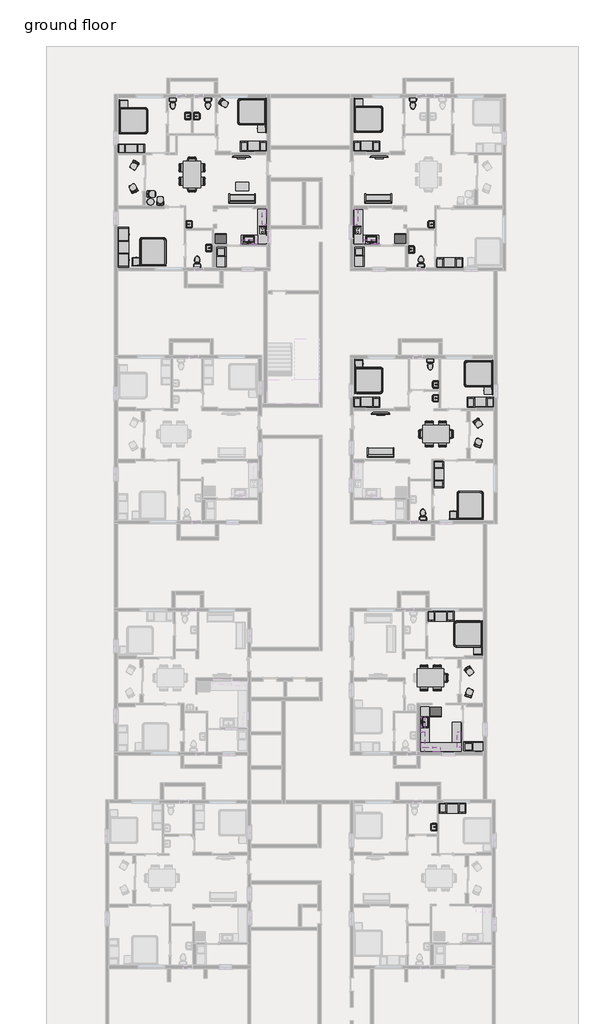
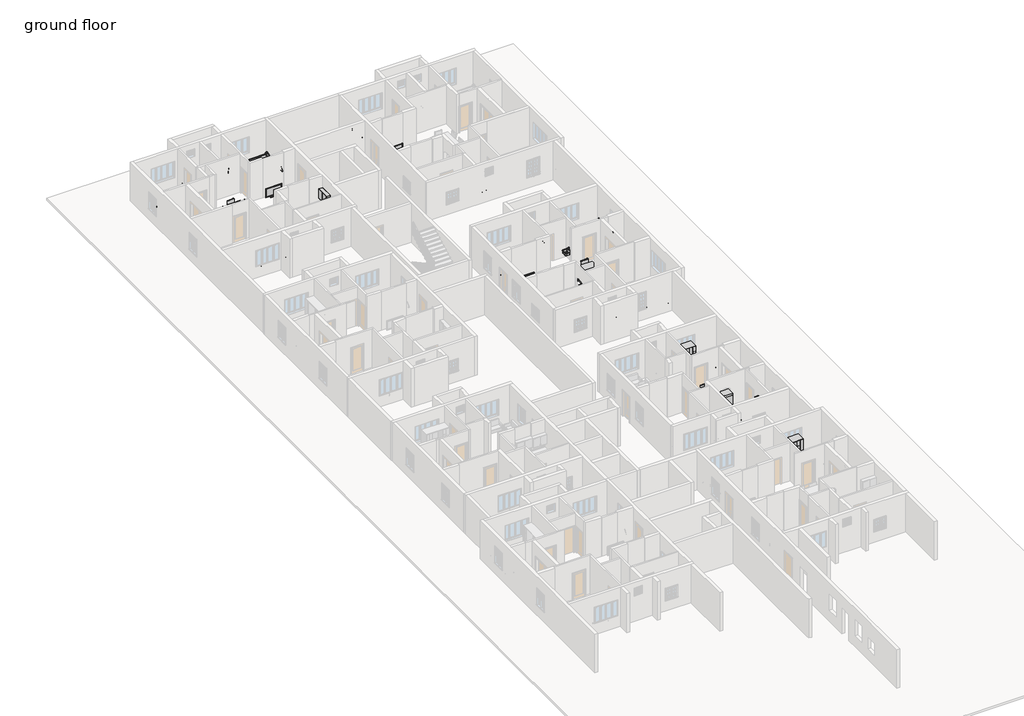
# One storey, part 13 of 16: 81 furniture elements, 19 flow terminals, 11 proxies.
"""IFC4 building model written with IfcOpenShell, lengths in millimetres."""

from ifc_helpers import new_model, si_unit, origin, place, context, project, spatial, transform, mapped, element, save
from components import proxy_84368fe0, proxy_40295e01, proxy_97c73763, proxy_19935bb1, proxy_76352e5b, proxy_1934c8a4, flow_terminal_4d548711, flow_terminal_3ac2e542, flow_terminal_8d9ea526, toilet_domestic_3d_toilet_domestic_3d_ba6479b0, toilet_domestic_3d_toilet_domestic_3d_30431060, bed_design_8999_bed_design_8999_9c973422, bed_design_8999_bed_design_8999_e911dec7, furniture_f87f75a4, furniture_a56de0b1, furniture_5ca60c7f, furniture_97fe820d, furniture_007fecef, chair_task_chair_task_b7f3823b, chair_task_arms_chair_task_arms_fa5a08ef, furniture_deb1c5d1, furniture_78fcf777, furniture_7591947b, furniture_03a15ce7, furniture_53e129a0, furniture_dd44345b, furniture_3d2ef6d7, furniture_88072bd9, furniture_1f19b6cd, furniture_eb3a3c23, furniture_4fdbbe14, furniture_57f9710a, furniture_0b81fedb, furniture_e479396c, furniture_0bcc43ae, furniture_9d41381f, furniture_9929ec1f, furniture_f73e1c42

model = new_model("IFC4")

# Units and contexts
model_context = context("Model", 3, world=origin())
ifc_project = project(units=[si_unit("LENGTHUNIT", "METRE", prefix="MILLI")], contexts=[model_context])

# Site, building, storey
site = spatial("IfcSite", under=ifc_project)
building = spatial("IfcBuilding", under=site)
storey = spatial("IfcBuildingStorey", under=building, Name="ground floor", Elevation=609.6)

# Proxies
placement = place(None, origin())
proxy_shape = proxy_84368fe0(model_context)
element("IfcBuildingElementProxy", 1, Name="Cook Top-2 Unit : 16\" x 22\"", ObjectType="Cook Top-2 Unit : 16\" x 22\"", at=placement, inside=storey, context=model_context, shape_type="MappedRepresentation", body=[
    mapped(proxy_shape, transform((53260.5312819, 41205.614288, 609.6), x_axis=(1.0, 0.0, 0.0), y_axis=(0.0, 1.0, 0.0), z_axis=(0.0, 0.0, 1.0))),
])
proxy_2_shape = proxy_40295e01(model_context)
element("IfcBuildingElementProxy", 2, Name="Cook Top-2 Unit : 16\" x 22\"", ObjectType="Cook Top-2 Unit : 16\" x 22\"", at=placement, inside=storey, context=model_context, shape_type="MappedRepresentation", body=[
    mapped(proxy_2_shape, transform((59966.1312819, 41205.614288, 609.6), x_axis=(-1.0, 0.0, 0.0), y_axis=(0.0, -1.0, 0.0), z_axis=(0.0, 0.0, 1.0))),
])
proxy_3_shape = proxy_97c73763(model_context)
element("IfcBuildingElementProxy", 3, Name="Dryer : 27\" x 25\" x 35\"", ObjectType="Dryer : 27\" x 25\" x 35\"", at=placement, inside=storey, context=model_context, shape_type="MappedRepresentation", body=[
    mapped(proxy_3_shape, transform((50190.0538966, 39449.1934981, 609.6), x_axis=(0.0, -1.0, 0.0), y_axis=(1.0, 0.0, 0.0), z_axis=(0.0, 0.0, 1.0))),
])
element("IfcBuildingElementProxy", 4, Name="Dryer : 27\" x 25\" x 35\"", ObjectType="Dryer : 27\" x 25\" x 35\"", at=placement, inside=storey, context=model_context, shape_type="MappedRepresentation", body=[
    mapped(proxy_3_shape, transform((59691.3278279, 39474.5934981, 609.6), x_axis=(0.0, -1.0, 0.0), y_axis=(1.0, 0.0, 0.0), z_axis=(0.0, 0.0, 1.0))),
])
element("IfcBuildingElementProxy", 5, Name="Dryer : 27\" x 25\" x 35\"", ObjectType="Dryer : 27\" x 25\" x 35\"", at=placement, inside=storey, context=model_context, shape_type="MappedRepresentation", body=[
    mapped(proxy_3_shape, transform((67812.0859463, 5399.7775766, 609.6), x_axis=(1.0, 0.0, 0.0), y_axis=(0.0, 1.0, 0.0), z_axis=(0.0, 0.0, 1.0))),
])
proxy_4_shape = proxy_19935bb1(model_context)
element("IfcBuildingElementProxy", 6, Name="Refrigerator-Built-in : 30\" x 24\" LH", ObjectType="Refrigerator-Built-in : 30\" x 24\" LH", at=placement, inside=storey, context=model_context, shape_type="MappedRepresentation", body=[
    mapped(proxy_4_shape, transform((65262.8133315, 8104.2496364, 609.6), x_axis=(1.0, 0.0, 0.0), y_axis=(0.0, 1.0, 0.0), z_axis=(0.0, 0.0, 1.0))),
])
proxy_5_shape = proxy_76352e5b(model_context)
element("IfcBuildingElementProxy", 7, Name="Refrigerator-Built-in : 30\" x 24\" LH", ObjectType="Refrigerator-Built-in : 30\" x 24\" LH", at=placement, inside=storey, context=model_context, shape_type="MappedRepresentation", body=[
    mapped(proxy_5_shape, transform((50460.1812819, 40629.665558, 609.6), x_axis=(1.0, 0.0, 0.0), y_axis=(0.0, 1.0, 0.0), z_axis=(0.0, 0.0, 1.0))),
])
element("IfcBuildingElementProxy", 8, Name="Refrigerator-Built-in : 30\" x 24\" LH", ObjectType="Refrigerator-Built-in : 30\" x 24\" LH", at=placement, inside=storey, context=model_context, shape_type="MappedRepresentation", body=[
    mapped(proxy_5_shape, transform((62806.2552131, 40629.665558, 609.6), x_axis=(1.0, 0.0, 0.0), y_axis=(0.0, 1.0, 0.0), z_axis=(0.0, 0.0, 1.0))),
])
proxy_6_shape = proxy_1934c8a4(model_context)
element("IfcBuildingElementProxy", 9, Name="Washer : 25\" x 25\" x 35\"", ObjectType="Washer : 25\" x 25\" x 35\"", at=placement, inside=storey, context=model_context, shape_type="MappedRepresentation", body=[
    mapped(proxy_6_shape, transform((50225.5653356, 40125.6235103, 609.6), x_axis=(0.0, -1.0, 0.0), y_axis=(1.0, 0.0, 0.0), z_axis=(0.0, 0.0, 1.0))),
])
element("IfcBuildingElementProxy", 10, Name="Washer : 25\" x 25\" x 35\"", ObjectType="Washer : 25\" x 25\" x 35\"", at=placement, inside=storey, context=model_context, shape_type="MappedRepresentation", body=[
    mapped(proxy_6_shape, transform((59726.8392669, 40151.0235103, 609.6), x_axis=(0.0, -1.0, 0.0), y_axis=(1.0, 0.0, 0.0), z_axis=(0.0, 0.0, 1.0))),
])
element("IfcBuildingElementProxy", 11, Name="Washer : 25\" x 25\" x 35\"", ObjectType="Washer : 25\" x 25\" x 35\"", at=placement, inside=storey, context=model_context, shape_type="MappedRepresentation", body=[
    mapped(proxy_6_shape, transform((67110.9973853, 5441.2075888, 609.6), x_axis=(1.0, 0.0, 0.0), y_axis=(0.0, 1.0, 0.0), z_axis=(0.0, 0.0, 1.0))),
])

# Flow terminals
flow_terminal_shape = flow_terminal_4d548711(model_context)
element("IfcFlowTerminal", 12, ObjectType="Sink Kitchen-Single : 30\" x 21\"", at=placement, inside=storey, context=model_context, shape_type="MappedRepresentation", body=[
    mapped(flow_terminal_shape, transform((52412.6205224, 40563.7497039, 609.6), x_axis=(-1.0, 0.0, 0.0), y_axis=(0.0, -1.0, 0.0), z_axis=(0.0, 0.0, 1.0))),
])
element("IfcFlowTerminal", 13, ObjectType="Sink Kitchen-Single : 30\" x 21\"", at=placement, inside=storey, context=model_context, shape_type="MappedRepresentation", body=[
    mapped(flow_terminal_shape, transform((64489.676683, 7368.8508246, 609.6), x_axis=(0.0, 1.0, 0.0), y_axis=(-1.0, 0.0, 0.0), z_axis=(0.0, 0.0, 1.0))),
])
flow_terminal_2_shape = flow_terminal_3ac2e542(model_context)
element("IfcFlowTerminal", 14, ObjectType="Sink Kitchen-Single : 30\" x 21\"", at=placement, inside=storey, context=model_context, shape_type="MappedRepresentation", body=[
    mapped(flow_terminal_2_shape, transform((60814.0420413, 40563.7497039, 609.6), x_axis=(1.0, 0.0, 0.0), y_axis=(0.0, 1.0, 0.0), z_axis=(0.0, 0.0, 1.0))),
])
flow_terminal_3_shape = flow_terminal_8d9ea526(model_context)
element("IfcFlowTerminal", 15, ObjectType="Sink Vanity-Square : 20\" x 18\"", at=placement, inside=storey, context=model_context, shape_type="MappedRepresentation", body=[
    mapped(flow_terminal_3_shape, transform((48234.5058086, 41623.6015966, 609.6), x_axis=(0.01205714691658211, 0.9999273099621953, 0.0), y_axis=(-0.9999273099621953, 0.01205714691658211, 0.0), z_axis=(0.0, 0.0, 1.0))),
])
element("IfcFlowTerminal", 16, ObjectType="Sink Vanity-Square : 20\" x 18\"", at=placement, inside=storey, context=model_context, shape_type="MappedRepresentation", body=[
    mapped(flow_terminal_3_shape, transform((49691.1133168, 40018.2935434, 609.6), x_axis=(0.0, -1.0, 0.0), y_axis=(1.0, 0.0, 0.0), z_axis=(0.0, 0.0, 1.0))),
])
element("IfcFlowTerminal", 17, ObjectType="Sink Vanity-Square : 20\" x 18\"", at=placement, inside=storey, context=model_context, shape_type="MappedRepresentation", body=[
    mapped(flow_terminal_3_shape, transform((48245.9195817, 49103.029965, 609.6), x_axis=(0.0, -1.0, 0.0), y_axis=(1.0, 0.0, 0.0), z_axis=(0.0, 0.0, 1.0))),
])
element("IfcFlowTerminal", 18, ObjectType="Sink Vanity-Square : 20\" x 18\"", at=placement, inside=storey, context=model_context, shape_type="MappedRepresentation", body=[
    mapped(flow_terminal_3_shape, transform((48755.0527323, 49063.0030585, 609.6), x_axis=(0.0, 1.0, 0.0), y_axis=(-1.0, 0.0, 0.0), z_axis=(0.0, 0.0, 1.0))),
])
element("IfcFlowTerminal", 19, ObjectType="Sink Vanity-Square : 20\" x 18\"", at=placement, inside=storey, context=model_context, shape_type="MappedRepresentation", body=[
    mapped(flow_terminal_3_shape, transform((64991.9370405, 41653.02877, 609.6), x_axis=(0.0, -1.0, 0.0), y_axis=(1.0, 0.0, 0.0), z_axis=(0.0, 0.0, 1.0))),
])
element("IfcFlowTerminal", 20, ObjectType="Sink Vanity-Square : 20\" x 18\"", at=placement, inside=storey, context=model_context, shape_type="MappedRepresentation", body=[
    mapped(flow_terminal_3_shape, transform((63532.9943061, 39880.7582649, 609.6), x_axis=(-0.012057146916551579, 0.9999273099621956, 0.0), y_axis=(-0.9999273099621956, -0.012057146916551579, 0.0), z_axis=(0.0, 0.0, 1.0))),
])
element("IfcFlowTerminal", 21, ObjectType="Sink Vanity-Square : 20\" x 18\"", at=placement, inside=storey, context=model_context, shape_type="MappedRepresentation", body=[
    mapped(flow_terminal_3_shape, transform((65297.7858807, 30630.1271371, 609.6), x_axis=(0.0, -1.0, 0.0), y_axis=(1.0, 0.0, 0.0), z_axis=(0.0, 0.0, 1.0))),
])
element("IfcFlowTerminal", 22, ObjectType="Sink Vanity-Square : 20\" x 18\"", at=placement, inside=storey, context=model_context, shape_type="MappedRepresentation", body=[
    mapped(flow_terminal_3_shape, transform((65297.7858807, 29682.8183877, 609.6), x_axis=(0.0, -1.0, 0.0), y_axis=(1.0, 0.0, 0.0), z_axis=(0.0, 0.0, 1.0))),
])
element("IfcFlowTerminal", 23, ObjectType="Sink Vanity-Square : 20\" x 18\"", at=placement, inside=storey, context=model_context, shape_type="MappedRepresentation", body=[
    mapped(flow_terminal_3_shape, transform((65183.4858807, 170.5278741, 609.6), x_axis=(0.0, -1.0, 0.0), y_axis=(1.0, 0.0, 0.0), z_axis=(0.0, 0.0, 1.0))),
])
toilet_domestic_3d_toilet_domestic_3d_shape = toilet_domestic_3d_toilet_domestic_3d_ba6479b0(model_context)
toilet_domestic_3d_toilet_domestic_3d_2_shape = toilet_domestic_3d_toilet_domestic_3d_30431060(model_context)
element("IfcFlowTerminal", 24, ObjectType="Toilet-Domestic-3D : Toilet-Domestic-3D", at=placement, inside=storey, context=model_context, shape_type="MappedRepresentation", body=[
    mapped(toilet_domestic_3d_toilet_domestic_3d_shape, transform((48837.5141396, 39156.8770141, 609.6), x_axis=(-1.0, 0.0, 0.0), y_axis=(0.0, -1.0, 0.0), z_axis=(0.0, 0.0, 1.0))),
    mapped(toilet_domestic_3d_toilet_domestic_3d_2_shape, transform((48837.5141396, 39156.8770141, 609.6), x_axis=(-1.0, 0.0, 0.0), y_axis=(0.0, -1.0, 0.0), z_axis=(0.0, 0.0, 1.0))),
])
element("IfcFlowTerminal", 25, ObjectType="Toilet-Domestic-3D : Toilet-Domestic-3D", at=placement, inside=storey, context=model_context, shape_type="MappedRepresentation", body=[
    mapped(toilet_domestic_3d_toilet_domestic_3d_shape, transform((49576.2011467, 49859.7430562, 609.6), x_axis=(1.0, 0.0, 0.0), y_axis=(0.0, 1.0, 0.0), z_axis=(0.0, 0.0, 1.0))),
    mapped(toilet_domestic_3d_toilet_domestic_3d_2_shape, transform((49576.2011467, 49859.7430562, 609.6), x_axis=(1.0, 0.0, 0.0), y_axis=(0.0, 1.0, 0.0), z_axis=(0.0, 0.0, 1.0))),
])
element("IfcFlowTerminal", 26, ObjectType="Toilet-Domestic-3D : Toilet-Domestic-3D", at=placement, inside=storey, context=model_context, shape_type="MappedRepresentation", body=[
    mapped(toilet_domestic_3d_toilet_domestic_3d_shape, transform((47154.8643084, 49859.7430562, 609.6), x_axis=(1.0, 0.0, 0.0), y_axis=(0.0, 1.0, 0.0), z_axis=(0.0, 0.0, 1.0))),
    mapped(toilet_domestic_3d_toilet_domestic_3d_2_shape, transform((47154.8643084, 49859.7430562, 609.6), x_axis=(1.0, 0.0, 0.0), y_axis=(0.0, 1.0, 0.0), z_axis=(0.0, 0.0, 1.0))),
])
element("IfcFlowTerminal", 27, ObjectType="Toilet-Domestic-3D : Toilet-Domestic-3D", at=placement, inside=storey, context=model_context, shape_type="MappedRepresentation", body=[
    mapped(toilet_domestic_3d_toilet_domestic_3d_shape, transform((63678.9871882, 49859.7430562, 609.6), x_axis=(1.0, 0.0, 0.0), y_axis=(0.0, 1.0, 0.0), z_axis=(0.0, 0.0, 1.0))),
    mapped(toilet_domestic_3d_toilet_domestic_3d_2_shape, transform((63678.9871882, 49859.7430562, 609.6), x_axis=(1.0, 0.0, 0.0), y_axis=(0.0, 1.0, 0.0), z_axis=(0.0, 0.0, 1.0))),
])
element("IfcFlowTerminal", 28, ObjectType="Toilet-Domestic-3D : Toilet-Domestic-3D", at=placement, inside=storey, context=model_context, shape_type="MappedRepresentation", body=[
    mapped(toilet_domestic_3d_toilet_domestic_3d_shape, transform((64239.5976633, 39156.8770141, 609.6), x_axis=(-1.0, 0.0, 0.0), y_axis=(0.0, -1.0, 0.0), z_axis=(0.0, 0.0, 1.0))),
    mapped(toilet_domestic_3d_toilet_domestic_3d_2_shape, transform((64239.5976633, 39156.8770141, 609.6), x_axis=(-1.0, 0.0, 0.0), y_axis=(0.0, -1.0, 0.0), z_axis=(0.0, 0.0, 1.0))),
])
element("IfcFlowTerminal", 29, ObjectType="Toilet-Domestic-3D : Toilet-Domestic-3D", at=placement, inside=storey, context=model_context, shape_type="MappedRepresentation", body=[
    mapped(toilet_domestic_3d_toilet_domestic_3d_shape, transform((64874.6812819, 31905.6690378, 609.6), x_axis=(1.0, 0.0, 0.0), y_axis=(0.0, 1.0, 0.0), z_axis=(0.0, 0.0, 1.0))),
    mapped(toilet_domestic_3d_toilet_domestic_3d_2_shape, transform((64874.6812819, 31905.6690378, 609.6), x_axis=(1.0, 0.0, 0.0), y_axis=(0.0, 1.0, 0.0), z_axis=(0.0, 0.0, 1.0))),
])
element("IfcFlowTerminal", 30, ObjectType="Toilet-Domestic-3D : Toilet-Domestic-3D", at=placement, inside=storey, context=model_context, shape_type="MappedRepresentation", body=[
    mapped(toilet_domestic_3d_toilet_domestic_3d_shape, transform((64368.0652737, 21744.4610925, 609.6), x_axis=(-1.0, 0.0, 0.0), y_axis=(0.0, -1.0, 0.0), z_axis=(0.0, 0.0, 1.0))),
    mapped(toilet_domestic_3d_toilet_domestic_3d_2_shape, transform((64368.0652737, 21744.4610925, 609.6), x_axis=(-1.0, 0.0, 0.0), y_axis=(0.0, -1.0, 0.0), z_axis=(0.0, 0.0, 1.0))),
])

# Furniture
bed_design_8999_bed_design_8999_shape = bed_design_8999_bed_design_8999_9c973422(model_context)
bed_design_8999_bed_design_8999_2_shape = bed_design_8999_bed_design_8999_e911dec7(model_context)
element("IfcFurniture", 31, ObjectType="BED_DESIGN_8999 : BED_DESIGN_8999", at=placement, inside=storey, context=model_context, shape_type="MappedRepresentation", body=[
    mapped(bed_design_8999_bed_design_8999_shape, transform((45592.726243, 40719.5817487, 609.6), x_axis=(-1.0, 0.0, 0.0), y_axis=(0.0, -1.0, 0.0), z_axis=(0.0, 0.0, 1.0))),
    mapped(bed_design_8999_bed_design_8999_2_shape, transform((45592.726243, 40719.5817487, 609.6), x_axis=(-1.0, 0.0, 0.0), y_axis=(0.0, -1.0, 0.0), z_axis=(0.0, 0.0, 1.0))),
])
element("IfcFurniture", 32, ObjectType="BED_DESIGN_8999 : BED_DESIGN_8999", at=placement, inside=storey, context=model_context, shape_type="MappedRepresentation", body=[
    mapped(bed_design_8999_bed_design_8999_shape, transform((45422.4680531, 48968.4210279, 609.6), x_axis=(0.0, 1.0, 0.0), y_axis=(-1.0, 0.0, 0.0), z_axis=(0.0, 0.0, 1.0))),
    mapped(bed_design_8999_bed_design_8999_2_shape, transform((45422.4680531, 48968.4210279, 609.6), x_axis=(0.0, 1.0, 0.0), y_axis=(-1.0, 0.0, 0.0), z_axis=(0.0, 0.0, 1.0))),
])
element("IfcFurniture", 33, ObjectType="BED_DESIGN_8999 : BED_DESIGN_8999", at=placement, inside=storey, context=model_context, shape_type="MappedRepresentation", body=[
    mapped(bed_design_8999_bed_design_8999_shape, transform((51628.3064817, 49188.0273256, 609.6), x_axis=(0.0, -1.0, 0.0), y_axis=(1.0, 0.0, 0.0), z_axis=(0.0, 0.0, 1.0))),
    mapped(bed_design_8999_bed_design_8999_2_shape, transform((51628.3064817, 49188.0273256, 609.6), x_axis=(0.0, -1.0, 0.0), y_axis=(1.0, 0.0, 0.0), z_axis=(0.0, 0.0, 1.0))),
])
element("IfcFurniture", 34, ObjectType="BED_DESIGN_8999 : BED_DESIGN_8999", at=placement, inside=storey, context=model_context, shape_type="MappedRepresentation", body=[
    mapped(bed_design_8999_bed_design_8999_shape, transform((61598.356082, 49071.7390836, 609.6), x_axis=(0.0, 1.0, 0.0), y_axis=(-1.0, 0.0, 0.0), z_axis=(0.0, 0.0, 1.0))),
    mapped(bed_design_8999_bed_design_8999_2_shape, transform((61598.356082, 49071.7390836, 609.6), x_axis=(0.0, 1.0, 0.0), y_axis=(-1.0, 0.0, 0.0), z_axis=(0.0, 0.0, 1.0))),
])
element("IfcFurniture", 35, ObjectType="BED_DESIGN_8999 : BED_DESIGN_8999", at=placement, inside=storey, context=model_context, shape_type="MappedRepresentation", body=[
    mapped(bed_design_8999_bed_design_8999_shape, transform((67217.8305199, 31152.027058, 609.6), x_axis=(0.0, -1.0, 0.0), y_axis=(1.0, 0.0, 0.0), z_axis=(0.0, 0.0, 1.0))),
    mapped(bed_design_8999_bed_design_8999_2_shape, transform((67217.8305199, 31152.027058, 609.6), x_axis=(0.0, -1.0, 0.0), y_axis=(1.0, 0.0, 0.0), z_axis=(0.0, 0.0, 1.0))),
])
element("IfcFurniture", 36, ObjectType="BED_DESIGN_8999 : BED_DESIGN_8999", at=placement, inside=storey, context=model_context, shape_type="MappedRepresentation", body=[
    mapped(bed_design_8999_bed_design_8999_shape, transform((61617.1320439, 31092.2650652, 609.6), x_axis=(0.0, 1.0, 0.0), y_axis=(-1.0, 0.0, 0.0), z_axis=(0.0, 0.0, 1.0))),
    mapped(bed_design_8999_bed_design_8999_2_shape, transform((61617.1320439, 31092.2650652, 609.6), x_axis=(0.0, 1.0, 0.0), y_axis=(-1.0, 0.0, 0.0), z_axis=(0.0, 0.0, 1.0))),
])
element("IfcFurniture", 37, ObjectType="BED_DESIGN_8999 : BED_DESIGN_8999", at=placement, inside=storey, context=model_context, shape_type="MappedRepresentation", body=[
    mapped(bed_design_8999_bed_design_8999_shape, transform((67418.6270735, 23281.7658272, 609.6), x_axis=(-1.0, 0.0, 0.0), y_axis=(0.0, -1.0, 0.0), z_axis=(0.0, 0.0, 1.0))),
    mapped(bed_design_8999_bed_design_8999_2_shape, transform((67418.6270735, 23281.7658272, 609.6), x_axis=(-1.0, 0.0, 0.0), y_axis=(0.0, -1.0, 0.0), z_axis=(0.0, 0.0, 1.0))),
])
element("IfcFurniture", 38, ObjectType="BED_DESIGN_8999 : BED_DESIGN_8999", at=placement, inside=storey, context=model_context, shape_type="MappedRepresentation", body=[
    mapped(bed_design_8999_bed_design_8999_shape, transform((66506.6312819, 13242.4150652, 609.6), x_axis=(0.0, -1.0, 0.0), y_axis=(1.0, 0.0, 0.0), z_axis=(0.0, 0.0, 1.0))),
    mapped(bed_design_8999_bed_design_8999_2_shape, transform((66506.6312819, 13242.4150652, 609.6), x_axis=(0.0, -1.0, 0.0), y_axis=(1.0, 0.0, 0.0), z_axis=(0.0, 0.0, 1.0))),
])
furniture_shape = furniture_f87f75a4(model_context)
element("IfcFurniture", 39, ObjectType="Base Cabinet-Combo01 : 30\"", at=placement, inside=storey, context=model_context, shape_type="MappedRepresentation", body=[
    mapped(furniture_shape, transform((53641.5312819, 42333.1553351, 609.6), x_axis=(0.0, -1.0, 0.0), y_axis=(1.0, 0.0, 0.0), z_axis=(0.0, 0.0, 1.0))),
])
element("IfcFurniture", 40, ObjectType="Base Cabinet-Combo01 : 30\"", at=placement, inside=storey, context=model_context, shape_type="MappedRepresentation", body=[
    mapped(furniture_shape, transform((53641.5312819, 41571.1553351, 609.6), x_axis=(0.0, -1.0, 0.0), y_axis=(1.0, 0.0, 0.0), z_axis=(0.0, 0.0, 1.0))),
])
element("IfcFurniture", 41, ObjectType="Base Cabinet-Combo01 : 30\"", at=placement, inside=storey, context=model_context, shape_type="MappedRepresentation", body=[
    mapped(furniture_shape, transform((67040.0312819, 6638.5160974, 609.6), x_axis=(0.0, -1.0, 0.0), y_axis=(1.0, 0.0, 0.0), z_axis=(0.0, 0.0, 1.0))),
])
element("IfcFurniture", 42, ObjectType="Base Cabinet-Combo01 : 30\"", at=placement, inside=storey, context=model_context, shape_type="MappedRepresentation", body=[
    mapped(furniture_shape, transform((64182.5312819, 6600.6273603, 609.6), x_axis=(0.0, 1.0, 0.0), y_axis=(-1.0, 0.0, 0.0), z_axis=(0.0, 0.0, 1.0))),
])
furniture_2_shape = furniture_a56de0b1(model_context)
element("IfcFurniture", 43, ObjectType="Base Cabinet-Combo01 : 30\"", at=placement, inside=storey, context=model_context, shape_type="MappedRepresentation", body=[
    mapped(furniture_2_shape, transform((59585.1312819, 42333.1553351, 609.6), x_axis=(0.0, -1.0, 0.0), y_axis=(1.0, 0.0, 0.0), z_axis=(0.0, 0.0, 1.0))),
])
element("IfcFurniture", 44, ObjectType="Base Cabinet-Combo01 : 30\"", at=placement, inside=storey, context=model_context, shape_type="MappedRepresentation", body=[
    mapped(furniture_2_shape, transform((59585.1312819, 41571.1553351, 609.6), x_axis=(0.0, -1.0, 0.0), y_axis=(1.0, 0.0, 0.0), z_axis=(0.0, 0.0, 1.0))),
])
furniture_3_shape = furniture_5ca60c7f(model_context)
element("IfcFurniture", 45, ObjectType="Base Cabinet-Combo01 : 30\" 2", at=placement, inside=storey, context=model_context, shape_type="MappedRepresentation", body=[
    mapped(furniture_3_shape, transform((65592.5435769, 5882.7650652, 609.6), x_axis=(1.0, 0.0, 0.0), y_axis=(0.0, 1.0, 0.0), z_axis=(0.0, 0.0, 1.0))),
])
furniture_4_shape = furniture_97fe820d(model_context)
element("IfcFurniture", 46, ObjectType="Base Cabinet-Corner Unit-Square : 36\"", at=placement, inside=storey, context=model_context, shape_type="MappedRepresentation", body=[
    mapped(furniture_4_shape, transform((53641.5312819, 40783.1307449, 609.6), x_axis=(0.0, -1.0, 0.0), y_axis=(1.0, 0.0, 0.0), z_axis=(0.0, 0.0, 1.0))),
])
element("IfcFurniture", 47, ObjectType="Base Cabinet-Corner Unit-Square : 36\"", at=placement, inside=storey, context=model_context, shape_type="MappedRepresentation", body=[
    mapped(furniture_4_shape, transform((67040.0312819, 5850.4915073, 609.6), x_axis=(0.0, -1.0, 0.0), y_axis=(1.0, 0.0, 0.0), z_axis=(0.0, 0.0, 1.0))),
])
element("IfcFurniture", 48, ObjectType="Base Cabinet-Corner Unit-Square : 36\"", at=placement, inside=storey, context=model_context, shape_type="MappedRepresentation", body=[
    mapped(furniture_4_shape, transform((64709.2689868, 5323.9650652, 609.6), x_axis=(-1.0, 0.0, 0.0), y_axis=(0.0, -1.0, 0.0), z_axis=(0.0, 0.0, 1.0))),
])
furniture_5_shape = furniture_007fecef(model_context)
element("IfcFurniture", 49, ObjectType="Base Cabinet-Corner Unit-Square : 36\"", at=placement, inside=storey, context=model_context, shape_type="MappedRepresentation", body=[
    mapped(furniture_5_shape, transform((59585.1312819, 40783.1307449, 609.6), x_axis=(0.0, -1.0, 0.0), y_axis=(1.0, 0.0, 0.0), z_axis=(0.0, 0.0, 1.0))),
])
chair_task_chair_task_shape = chair_task_chair_task_b7f3823b(model_context)
element("IfcFurniture", 50, ObjectType="Chair-Task : Chair-Task", at=placement, inside=storey, context=model_context, shape_type="MappedRepresentation", body=[
    mapped(chair_task_chair_task_shape, transform((47851.04103, 45663.0104868, 609.6), x_axis=(0.0, -1.0, 0.0), y_axis=(1.0, 0.0, 0.0), z_axis=(0.0, 0.0, 1.0))),
])
element("IfcFurniture", 51, ObjectType="Chair-Task : Chair-Task", at=placement, inside=storey, context=model_context, shape_type="MappedRepresentation", body=[
    mapped(chair_task_chair_task_shape, transform((49108.1328332, 45381.0288474, 609.6), x_axis=(0.0, 1.0, 0.0), y_axis=(-1.0, 0.0, 0.0), z_axis=(0.0, 0.0, 1.0))),
])
element("IfcFurniture", 52, ObjectType="Chair-Task : Chair-Task", at=placement, inside=storey, context=model_context, shape_type="MappedRepresentation", body=[
    mapped(chair_task_chair_task_shape, transform((47851.04103, 44748.6104868, 609.6), x_axis=(0.0, -1.0, 0.0), y_axis=(1.0, 0.0, 0.0), z_axis=(0.0, 0.0, 1.0))),
])
element("IfcFurniture", 53, ObjectType="Chair-Task : Chair-Task", at=placement, inside=storey, context=model_context, shape_type="MappedRepresentation", body=[
    mapped(chair_task_chair_task_shape, transform((49108.1328332, 44466.6288474, 609.6), x_axis=(0.0, 1.0, 0.0), y_axis=(-1.0, 0.0, 0.0), z_axis=(0.0, 0.0, 1.0))),
])
element("IfcFurniture", 54, ObjectType="Chair-Task : Chair-Task", at=placement, inside=storey, context=model_context, shape_type="MappedRepresentation", body=[
    mapped(chair_task_chair_task_shape, transform((64663.8404622, 26580.5700511, 609.6), x_axis=(1.0, 0.0, 0.0), y_axis=(0.0, 1.0, 0.0), z_axis=(0.0, 0.0, 1.0))),
])
element("IfcFurniture", 55, ObjectType="Chair-Task : Chair-Task", at=placement, inside=storey, context=model_context, shape_type="MappedRepresentation", body=[
    mapped(chair_task_chair_task_shape, transform((64945.8221015, 27837.6618544, 609.6), x_axis=(-1.0, 0.0, 0.0), y_axis=(0.0, -1.0, 0.0), z_axis=(0.0, 0.0, 1.0))),
])
element("IfcFurniture", 56, ObjectType="Chair-Task : Chair-Task", at=placement, inside=storey, context=model_context, shape_type="MappedRepresentation", body=[
    mapped(chair_task_chair_task_shape, transform((65578.2404622, 26580.5700511, 609.6), x_axis=(1.0, 0.0, 0.0), y_axis=(0.0, 1.0, 0.0), z_axis=(0.0, 0.0, 1.0))),
])
element("IfcFurniture", 57, ObjectType="Chair-Task : Chair-Task", at=placement, inside=storey, context=model_context, shape_type="MappedRepresentation", body=[
    mapped(chair_task_chair_task_shape, transform((65860.2221015, 27837.6618544, 609.6), x_axis=(-1.0, 0.0, 0.0), y_axis=(0.0, -1.0, 0.0), z_axis=(0.0, 0.0, 1.0))),
])
element("IfcFurniture", 58, ObjectType="Chair-Task : Chair-Task", at=placement, inside=storey, context=model_context, shape_type="MappedRepresentation", body=[
    mapped(chair_task_chair_task_shape, transform((64590.2221015, 11057.9109668, 609.6), x_axis=(-1.0, 0.0, 0.0), y_axis=(0.0, -1.0, 0.0), z_axis=(0.0, 0.0, 1.0))),
])
element("IfcFurniture", 59, ObjectType="Chair-Task : Chair-Task", at=placement, inside=storey, context=model_context, shape_type="MappedRepresentation", body=[
    mapped(chair_task_chair_task_shape, transform((65222.6404622, 9800.8191635, 609.6), x_axis=(1.0, 0.0, 0.0), y_axis=(0.0, 1.0, 0.0), z_axis=(0.0, 0.0, 1.0))),
])
element("IfcFurniture", 60, ObjectType="Chair-Task : Chair-Task", at=placement, inside=storey, context=model_context, shape_type="MappedRepresentation", body=[
    mapped(chair_task_chair_task_shape, transform((65504.6221015, 11057.9109668, 609.6), x_axis=(-1.0, 0.0, 0.0), y_axis=(0.0, -1.0, 0.0), z_axis=(0.0, 0.0, 1.0))),
])
element("IfcFurniture", 61, ObjectType="Chair-Task : Chair-Task", at=placement, inside=storey, context=model_context, shape_type="MappedRepresentation", body=[
    mapped(chair_task_chair_task_shape, transform((64308.2404622, 9800.8191635, 609.6), x_axis=(1.0, 0.0, 0.0), y_axis=(0.0, 1.0, 0.0), z_axis=(0.0, 0.0, 1.0))),
])
chair_task_arms_chair_task_arms_shape = chair_task_arms_chair_task_arms_fa5a08ef(model_context)
element("IfcFurniture", 62, ObjectType="Chair-Task Arms : Chair-Task Arms", at=placement, inside=storey, context=model_context, shape_type="MappedRepresentation", body=[
    mapped(chair_task_arms_chair_task_arms_shape, transform((48338.5961119, 44131.4737655, 609.6), x_axis=(1.0, 0.0, 0.0), y_axis=(0.0, 1.0, 0.0), z_axis=(0.0, 0.0, 1.0))),
])
element("IfcFurniture", 63, ObjectType="Chair-Task Arms : Chair-Task Arms", at=placement, inside=storey, context=model_context, shape_type="MappedRepresentation", body=[
    mapped(chair_task_arms_chair_task_arms_shape, transform((48620.5777513, 45998.1655688, 609.6), x_axis=(-1.0, 0.0, 0.0), y_axis=(0.0, -1.0, 0.0), z_axis=(0.0, 0.0, 1.0))),
])
element("IfcFurniture", 64, ObjectType="Chair-Task Arms : Chair-Task Arms", at=placement, inside=storey, context=model_context, shape_type="MappedRepresentation", body=[
    mapped(chair_task_arms_chair_task_arms_shape, transform((66195.3771835, 27068.1251331, 609.6), x_axis=(0.0, 1.0, 0.0), y_axis=(-1.0, 0.0, 0.0), z_axis=(0.0, 0.0, 1.0))),
])
element("IfcFurniture", 65, ObjectType="Chair-Task Arms : Chair-Task Arms", at=placement, inside=storey, context=model_context, shape_type="MappedRepresentation", body=[
    mapped(chair_task_arms_chair_task_arms_shape, transform((64328.6853802, 27350.1067724, 609.6), x_axis=(0.0, -1.0, 0.0), y_axis=(1.0, 0.0, 0.0), z_axis=(0.0, 0.0, 1.0))),
])
element("IfcFurniture", 66, ObjectType="Chair-Task Arms : Chair-Task Arms", at=placement, inside=storey, context=model_context, shape_type="MappedRepresentation", body=[
    mapped(chair_task_arms_chair_task_arms_shape, transform((65839.7771835, 10288.3742455, 609.6), x_axis=(0.0, 1.0, 0.0), y_axis=(-1.0, 0.0, 0.0), z_axis=(0.0, 0.0, 1.0))),
])
furniture_6_shape = furniture_deb1c5d1(model_context)
element("IfcFurniture", 67, ObjectType="Counter Top : 24\" Depth", at=placement, inside=storey, context=model_context, shape_type="MappedRepresentation", body=[
    mapped(furniture_6_shape, transform((53641.5312819, 41494.3307449, 609.6), x_axis=(0.0, -1.0, 0.0), y_axis=(1.0, 0.0, 0.0), z_axis=(0.0, 0.0, 1.0))),
])
furniture_7_shape = furniture_78fcf777(model_context)
element("IfcFurniture", 68, ObjectType="Counter Top : 24\" Depth", at=placement, inside=storey, context=model_context, shape_type="MappedRepresentation", body=[
    mapped(furniture_7_shape, transform((59585.1312819, 41494.3307449, 609.6), x_axis=(0.0, -1.0, 0.0), y_axis=(1.0, 0.0, 0.0), z_axis=(0.0, 0.0, 1.0))),
])
furniture_8_shape = furniture_7591947b(model_context)
element("IfcFurniture", 69, ObjectType="Counter Top : 24\" Depth", at=placement, inside=storey, context=model_context, shape_type="MappedRepresentation", body=[
    mapped(furniture_8_shape, transform((65839.5689868, 5323.9650652, 609.6), x_axis=(-1.0, 0.0, 0.0), y_axis=(0.0, -1.0, 0.0), z_axis=(0.0, 0.0, 1.0))),
])
furniture_9_shape = furniture_03a15ce7(model_context)
element("IfcFurniture", 70, ObjectType="Counter Top : 24\" Depth", at=placement, inside=storey, context=model_context, shape_type="MappedRepresentation", body=[
    mapped(furniture_9_shape, transform((67040.0312819, 6183.5829524, 609.6), x_axis=(0.0, -1.0, 0.0), y_axis=(1.0, 0.0, 0.0), z_axis=(0.0, 0.0, 1.0))),
])
furniture_10_shape = furniture_53e129a0(model_context)
element("IfcFurniture", 71, ObjectType="Counter Top w Sink Hole : 24\" Depth", at=placement, inside=storey, context=model_context, shape_type="MappedRepresentation", body=[
    mapped(furniture_10_shape, transform((51806.0689868, 40256.6043028, 609.6), x_axis=(-1.0, 0.0, 0.0), y_axis=(0.0, -1.0, 0.0), z_axis=(0.0, 0.0, 1.0))),
])
furniture_11_shape = furniture_dd44345b(model_context)
element("IfcFurniture", 72, ObjectType="Counter Top w Sink Hole : 24\" Depth", at=placement, inside=storey, context=model_context, shape_type="MappedRepresentation", body=[
    mapped(furniture_11_shape, transform((61420.5935769, 40256.6043028, 609.6), x_axis=(1.0, 0.0, 0.0), y_axis=(0.0, 1.0, 0.0), z_axis=(0.0, 0.0, 1.0))),
])
furniture_12_shape = furniture_3d2ef6d7(model_context)
element("IfcFurniture", 73, ObjectType="Counter Top w Sink Hole : 24\" Depth", at=placement, inside=storey, context=model_context, shape_type="MappedRepresentation", body=[
    mapped(furniture_12_shape, transform((64182.5312819, 7159.4273603, 609.6), x_axis=(0.0, 1.0, 0.0), y_axis=(-1.0, 0.0, 0.0), z_axis=(0.0, 0.0, 1.0))),
])
furniture_13_shape = furniture_88072bd9(model_context)
element("IfcFurniture", 74, ObjectType="Entertainment Center : 72\" x 72\" x 24\"", at=placement, inside=storey, context=model_context, shape_type="MappedRepresentation", body=[
    mapped(furniture_13_shape, transform((44304.8672911, 47259.2810851, 609.6), x_axis=(1.0, 0.0, 0.0), y_axis=(0.0, 1.0, 0.0), z_axis=(0.0, 0.0, 1.0))),
])
element("IfcFurniture", 75, ObjectType="Entertainment Center : 72\" x 72\" x 24\"", at=placement, inside=storey, context=model_context, shape_type="MappedRepresentation", body=[
    mapped(furniture_13_shape, transform((52727.1312819, 46560.6632967, 609.6), x_axis=(-1.0, 0.0, 0.0), y_axis=(0.0, -1.0, 0.0), z_axis=(0.0, 0.0, 1.0))),
])
element("IfcFurniture", 76, ObjectType="Entertainment Center : 72\" x 72\" x 24\"", at=placement, inside=storey, context=model_context, shape_type="MappedRepresentation", body=[
    mapped(furniture_13_shape, transform((60499.5312819, 46564.1897902, 609.6), x_axis=(-1.0, 0.0, 0.0), y_axis=(0.0, -1.0, 0.0), z_axis=(0.0, 0.0, 1.0))),
])
element("IfcFurniture", 77, ObjectType="Entertainment Center : 72\" x 72\" x 24\"", at=placement, inside=storey, context=model_context, shape_type="MappedRepresentation", body=[
    mapped(furniture_13_shape, transform((66199.9257323, 38560.5809867, 609.6), x_axis=(-1.0, 0.0, 0.0), y_axis=(0.0, -1.0, 0.0), z_axis=(0.0, 0.0, 1.0))),
])
element("IfcFurniture", 78, ObjectType="Entertainment Center : 72\" x 72\" x 24\"", at=placement, inside=storey, context=model_context, shape_type="MappedRepresentation", body=[
    mapped(furniture_13_shape, transform((68335.4312819, 28945.9650652, 609.6), x_axis=(-1.0, 0.0, 0.0), y_axis=(0.0, -1.0, 0.0), z_axis=(0.0, 0.0, 1.0))),
])
element("IfcFurniture", 79, ObjectType="Entertainment Center : 72\" x 72\" x 24\"", at=placement, inside=storey, context=model_context, shape_type="MappedRepresentation", body=[
    mapped(furniture_13_shape, transform((60499.5312819, 28945.9650652, 609.6), x_axis=(-1.0, 0.0, 0.0), y_axis=(0.0, -1.0, 0.0), z_axis=(0.0, 0.0, 1.0))),
])
element("IfcFurniture", 80, ObjectType="Entertainment Center : 72\" x 72\" x 24\"", at=placement, inside=storey, context=model_context, shape_type="MappedRepresentation", body=[
    mapped(furniture_13_shape, transform((65021.9112421, 24437.4650652, 609.6), x_axis=(0.0, 1.0, 0.0), y_axis=(-1.0, 0.0, 0.0), z_axis=(0.0, 0.0, 1.0))),
])
element("IfcFurniture", 81, ObjectType="Entertainment Center : 72\" x 72\" x 24\"", at=placement, inside=storey, context=model_context, shape_type="MappedRepresentation", body=[
    mapped(furniture_13_shape, transform((65604.9312819, 15102.9650652, 609.6), x_axis=(1.0, 0.0, 0.0), y_axis=(0.0, 1.0, 0.0), z_axis=(0.0, 0.0, 1.0))),
])
element("IfcFurniture", 82, ObjectType="Entertainment Center : 72\" x 72\" x 24\"", at=placement, inside=storey, context=model_context, shape_type="MappedRepresentation", body=[
    mapped(furniture_13_shape, transform((66405.0312819, 1901.0886336, 609.6), x_axis=(1.0, 0.0, 0.0), y_axis=(0.0, 1.0, 0.0), z_axis=(0.0, 0.0, 1.0))),
])
furniture_14_shape = furniture_1f19b6cd(model_context)
element("IfcFurniture", 83, ObjectType="Entertainment Center : 96\" x 84\" x 30\"", at=placement, inside=storey, context=model_context, shape_type="MappedRepresentation", body=[
    mapped(furniture_14_shape, transform((43357.1061463, 40059.1809867, 609.6), x_axis=(0.0, 1.0, 0.0), y_axis=(-1.0, 0.0, 0.0), z_axis=(0.0, 0.0, 1.0))),
])
furniture_15_shape = furniture_eb3a3c23(model_context)
element("IfcFurniture", 84, ObjectType="Seating-Auditorium : 18\" x 24\" x 30\"", at=placement, inside=storey, context=model_context, shape_type="MappedRepresentation", body=[
    mapped(furniture_15_shape, transform((45471.6114215, 43881.5911655, 609.6), x_axis=(0.0, -1.0, 0.0), y_axis=(1.0, 0.0, 0.0), z_axis=(0.0, 0.0, 1.0))),
])
element("IfcFurniture", 85, ObjectType="Seating-Auditorium : 18\" x 24\" x 30\"", at=placement, inside=storey, context=model_context, shape_type="MappedRepresentation", body=[
    mapped(furniture_15_shape, transform((46135.7589625, 43031.9676302, 609.6), x_axis=(1.0, 0.0, 0.0), y_axis=(0.0, 1.0, 0.0), z_axis=(0.0, 0.0, 1.0))),
])
element("IfcFurniture", 86, ObjectType="Seating-Auditorium : 18\" x 24\" x 30\"", at=placement, inside=storey, context=model_context, shape_type="MappedRepresentation", body=[
    mapped(furniture_15_shape, transform((44751.7812625, 45796.5068331, 609.6), x_axis=(-0.8660254037844514, 0.499999999999978, 0.0), y_axis=(-0.499999999999978, -0.8660254037844514, 0.0), z_axis=(0.0, 0.0, 1.0))),
])
element("IfcFurniture", 87, ObjectType="Seating-Auditorium : 18\" x 24\" x 30\"", at=placement, inside=storey, context=model_context, shape_type="MappedRepresentation", body=[
    mapped(furniture_15_shape, transform((44391.6003424, 43845.277646, 609.6), x_axis=(0.8974056171641766, 0.4412064803265965, 0.0), y_axis=(-0.4412064803265965, 0.8974056171641766, 0.0), z_axis=(0.0, 0.0, 1.0))),
])
element("IfcFurniture", 88, ObjectType="Seating-Auditorium : 18\" x 24\" x 30\"", at=placement, inside=storey, context=model_context, shape_type="MappedRepresentation", body=[
    mapped(furniture_15_shape, transform((50576.3864531, 50227.673469, 609.6), x_axis=(-0.5525353591441295, -0.8334894581789669, 0.0), y_axis=(0.8334894581789669, -0.5525353591441295, 0.0), z_axis=(0.0, 0.0, 1.0))),
])
furniture_16_shape = furniture_4fdbbe14(model_context)
element("IfcFurniture", 89, ObjectType="Seating-Auditorium : 18\" x 24\" x 30\"", at=placement, inside=storey, context=model_context, shape_type="MappedRepresentation", body=[
    mapped(furniture_16_shape, transform((67308.2233239, 10965.5390057, 609.6), x_axis=(0.8090169943749633, 0.5877852522924515, 0.0), y_axis=(-0.5877852522924515, 0.8090169943749633, 0.0), z_axis=(0.0, 0.0, 1.0))),
])
element("IfcFurniture", 90, ObjectType="Seating-Auditorium : 18\" x 24\" x 30\"", at=placement, inside=storey, context=model_context, shape_type="MappedRepresentation", body=[
    mapped(furniture_16_shape, transform((67641.7901237, 9138.8480143, 609.6), x_axis=(-0.9386081706685208, 0.3449850749732413, 0.0), y_axis=(-0.3449850749732413, -0.9386081706685208, 0.0), z_axis=(0.0, 0.0, 1.0))),
])
element("IfcFurniture", 91, ObjectType="Seating-Auditorium : 18\" x 24\" x 30\"", at=placement, inside=storey, context=model_context, shape_type="MappedRepresentation", body=[
    mapped(furniture_16_shape, transform((67909.2345365, 28023.848316, 609.6), x_axis=(0.8090169943749633, 0.5877852522924515, 0.0), y_axis=(-0.5877852522924515, 0.8090169943749633, 0.0), z_axis=(0.0, 0.0, 1.0))),
])
element("IfcFurniture", 92, ObjectType="Seating-Auditorium : 18\" x 24\" x 30\"", at=placement, inside=storey, context=model_context, shape_type="MappedRepresentation", body=[
    mapped(furniture_16_shape, transform((68268.2013364, 26349.5573246, 609.6), x_axis=(-0.9386081706685208, 0.3449850749732413, 0.0), y_axis=(-0.3449850749732413, -0.9386081706685208, 0.0), z_axis=(0.0, 0.0, 1.0))),
])
furniture_17_shape = furniture_57f9710a(model_context)
element("IfcFurniture", 93, ObjectType="Sofa : 72\"", at=placement, inside=storey, context=model_context, shape_type="MappedRepresentation", body=[
    mapped(furniture_17_shape, transform((52000.9619245, 43549.2255336, 609.6), x_axis=(-1.0, 0.0, 0.0), y_axis=(0.0, -1.0, 0.0), z_axis=(0.0, 0.0, 1.0))),
])
element("IfcFurniture", 94, ObjectType="Sofa : 72\"", at=placement, inside=storey, context=model_context, shape_type="MappedRepresentation", body=[
    mapped(furniture_17_shape, transform((61366.4416228, 43549.2255336, 609.6), x_axis=(-1.0, 0.0, 0.0), y_axis=(0.0, -1.0, 0.0), z_axis=(0.0, 0.0, 1.0))),
])
element("IfcFurniture", 95, ObjectType="Sofa : 72\"", at=placement, inside=storey, context=model_context, shape_type="MappedRepresentation", body=[
    mapped(furniture_17_shape, transform((61529.4121756, 26091.0193671, 609.6), x_axis=(-1.0, 0.0, 0.0), y_axis=(0.0, -1.0, 0.0), z_axis=(0.0, 0.0, 1.0))),
])
furniture_18_shape = furniture_0b81fedb(model_context)
element("IfcFurniture", 96, ObjectType="TV - Flat Screen : 50\"", at=placement, inside=storey, context=model_context, shape_type="MappedRepresentation", body=[
    mapped(furniture_18_shape, transform((51880.175796, 46311.6615304, 609.6), x_axis=(1.0, 0.0, 0.0), y_axis=(0.0, 1.0, 0.0), z_axis=(0.0, 0.0, 1.0))),
])
element("IfcFurniture", 97, ObjectType="TV - Flat Screen : 50\"", at=placement, inside=storey, context=model_context, shape_type="MappedRepresentation", body=[
    mapped(furniture_18_shape, transform((61363.9262496, 46311.7473534, 609.6), x_axis=(1.0, 0.0, 0.0), y_axis=(0.0, 1.0, 0.0), z_axis=(0.0, 0.0, 1.0))),
])
element("IfcFurniture", 98, ObjectType="TV - Flat Screen : 50\"", at=placement, inside=storey, context=model_context, shape_type="MappedRepresentation", body=[
    mapped(furniture_18_shape, transform((61462.986198, 28640.3330139, 609.6), x_axis=(1.0, 0.0, 0.0), y_axis=(0.0, 1.0, 0.0), z_axis=(0.0, 0.0, 1.0))),
])
furniture_19_shape = furniture_e479396c(model_context)
element("IfcFurniture", 99, ObjectType="Table-Coffee Rectangular : 48\" x 24\"", at=placement, inside=storey, context=model_context, shape_type="MappedRepresentation", body=[
    mapped(furniture_19_shape, transform((51319.7966371, 43874.2268908, 609.6), x_axis=(1.0, 0.0, 0.0), y_axis=(0.0, 1.0, 0.0), z_axis=(0.0, 0.0, 1.0))),
])
furniture_20_shape = furniture_0bcc43ae(model_context)
element("IfcFurniture", 100, ObjectType="Table-Conference2 w Chairs : 48\" x 144\"", at=placement, inside=storey, context=model_context, shape_type="MappedRepresentation", body=[
    mapped(furniture_20_shape, transform((48479.5869316, 45064.8196671, 609.6), x_axis=(0.0, 1.0, 0.0), y_axis=(-1.0, 0.0, 0.0), z_axis=(0.0, 0.0, 1.0))),
])
element("IfcFurniture", 101, ObjectType="Table-Conference2 w Chairs : 48\" x 144\"", at=placement, inside=storey, context=model_context, shape_type="MappedRepresentation", body=[
    mapped(furniture_20_shape, transform((65262.0312819, 27209.1159527, 609.6), x_axis=(-1.0, 0.0, 0.0), y_axis=(0.0, -1.0, 0.0), z_axis=(0.0, 0.0, 1.0))),
])
element("IfcFurniture", 102, ObjectType="Table-Conference2 w Chairs : dining table", at=placement, inside=storey, context=model_context, shape_type="MappedRepresentation", body=[
    mapped(furniture_20_shape, transform((64906.4312819, 10429.3650652, 609.6), x_axis=(-1.0, 0.0, 0.0), y_axis=(0.0, -1.0, 0.0), z_axis=(0.0, 0.0, 1.0))),
])
furniture_21_shape = furniture_9d41381f(model_context)
element("IfcFurniture", 103, ObjectType="Table-Trio End : 20\" Diameter", at=placement, inside=storey, context=model_context, shape_type="MappedRepresentation", body=[
    mapped(furniture_21_shape, transform((45625.5966479, 43186.5437743, 609.6), x_axis=(1.0, 0.0, 0.0), y_axis=(0.0, 1.0, 0.0), z_axis=(0.0, 0.0, 1.0))),
])
furniture_22_shape = furniture_9929ec1f(model_context)
element("IfcFurniture", 104, ObjectType="Upper Cabinet-Double Door-Wall : 42\"", at=placement, inside=storey, context=model_context, shape_type="MappedRepresentation", body=[
    mapped(furniture_22_shape, transform((53755.8312819, 42118.9218772, 704.85), x_axis=(0.0, 1.0, 0.0), y_axis=(-1.0, 0.0, 0.0), z_axis=(0.0, 0.0, 1.0))),
])
element("IfcFurniture", 105, ObjectType="Upper Cabinet-Double Door-Wall : 42\"", at=placement, inside=storey, context=model_context, shape_type="MappedRepresentation", body=[
    mapped(furniture_22_shape, transform((59470.8312819, 42160.7509295, 609.6), x_axis=(0.0, -1.0, 0.0), y_axis=(1.0, 0.0, 0.0), z_axis=(0.0, 0.0, 1.0))),
])
element("IfcFurniture", 106, ObjectType="Upper Cabinet-Double Door-Wall : 42\"", at=placement, inside=storey, context=model_context, shape_type="MappedRepresentation", body=[
    mapped(furniture_22_shape, transform((64068.2312819, 7252.386228, 609.6), x_axis=(0.0, -1.0, 0.0), y_axis=(1.0, 0.0, 0.0), z_axis=(0.0, 0.0, 1.0))),
])
element("IfcFurniture", 107, ObjectType="Upper Cabinet-Double Door-Wall : 42\"", at=placement, inside=storey, context=model_context, shape_type="MappedRepresentation", body=[
    mapped(furniture_22_shape, transform((64068.2312819, 6179.236228, 609.6), x_axis=(0.0, -1.0, 0.0), y_axis=(1.0, 0.0, 0.0), z_axis=(0.0, 0.0, 1.0))),
])
element("IfcFurniture", 108, ObjectType="Upper Cabinet-Double Door-Wall : 42\"", at=placement, inside=storey, context=model_context, shape_type="MappedRepresentation", body=[
    mapped(furniture_22_shape, transform((65003.6601191, 5209.6650652, 609.6), x_axis=(1.0, 0.0, 0.0), y_axis=(0.0, 1.0, 0.0), z_axis=(0.0, 0.0, 1.0))),
])
furniture_23_shape = furniture_f73e1c42(model_context)
element("IfcFurniture", 109, ObjectType="Upper Cabinet-Double Door-Wall : 42\"", at=placement, inside=storey, context=model_context, shape_type="MappedRepresentation", body=[
    mapped(furniture_23_shape, transform((52394.1875552, 40199.4543028, 609.6), x_axis=(1.0, 0.0, 0.0), y_axis=(0.0, 1.0, 0.0), z_axis=(0.0, 0.0, 1.0))),
])
element("IfcFurniture", 110, ObjectType="Upper Cabinet-Double Door-Wall : 42\"", at=placement, inside=storey, context=model_context, shape_type="MappedRepresentation", body=[
    mapped(furniture_23_shape, transform((60781.8020007, 40199.4543028, 609.6), x_axis=(1.0, 0.0, 0.0), y_axis=(0.0, 1.0, 0.0), z_axis=(0.0, 0.0, 1.0))),
])
element("IfcFurniture", 111, ObjectType="Upper Cabinet-Double Door-Wall : 42\"", at=placement, inside=storey, context=model_context, shape_type="MappedRepresentation", body=[
    mapped(furniture_23_shape, transform((67097.1812819, 6170.4939024, 609.6), x_axis=(0.0, 1.0, 0.0), y_axis=(-1.0, 0.0, 0.0), z_axis=(0.0, 0.0, 1.0))),
])

save(model, "model.ifc")

# Revit data of these elements
# Type "Cook Top-2 Unit : 16\" x 22\""
#   Assembly Code = "E1090400"
#   Counter Height = 3' - 0"
#   Depth = 1' - 10"
#   Width = 1' - 6"
#   Burner Material = Metal - Chrome
#   Cooktop Material = Metal - Steel, Polished
#   Default Elevation = 0
# Type "Dryer : 27\" x 25\" x 35\""
#   Label = "D"
#   Assembly Code = "E1090400"
#   Depth = 2' - 1"
#   Height = 2' - 11"
#   Width = 2' - 3"
#   Dryer Material = Metal - Paint Finish - Ivory,Glossy
#   Default Elevation = 0
# Type "Refrigerator-Built-in : 30\" x 24\" LH"
#   Assembly Code = "E1090400"
#   Depth = 2' - 0"
#   Handle = 0' - 0 1/4"
#   Height = 7' - 0"
#   Top Door Height = 5' - 0"
#   Width = 2' - 5 1/2"
#   Material = Metal - Paint Finish - Ivory,Glossy
#   Default Elevation = 0
# Type "Washer : 25\" x 25\" x 35\""
#   Label = "W"
#   Assembly Code = "E1090400"
#   Depth = 2' - 1"
#   Height = 2' - 11"
#   Width = 2' - 1"
#   Washer Material = Metal - Paint Finish - Ivory,Matte
#   Default Elevation = 0
# Type "Sink Kitchen-Single : 30\" x 21\""
#   Assembly Code = "D2010410"
#   Counter Height = 3' - 0"
#   Depth = 1' - 9"
#   Width = 2' - 6"
#   Faucet Material = Steel, Polished
#   Sink Material = Steel, Polished
#   Default Elevation = 0
# Type "Sink Vanity-Square : 20\" x 18\""
#   Assembly Code = "D2010400"
#   Counter Height = 2' - 7"
#   Depth = 1' - 6"
#   Width = 1' - 8"
#   Basin Material = Porcelain, Linen
#   Faucet Material = Steel, Polished
#   Default Elevation = 0
# Type "Toilet-Domestic-3D : Toilet-Domestic-3D"
#   Assembly Code = "D2010110"
#   Toilet - Bowl/Basin Material = Porcelain, Linen
#   Toilet - Seat Material = Laminate, Linen, Matte
#   Default Elevation = 0
# Type "BED_DESIGN_8999 : BED_DESIGN_8999"
#   Default Elevation = 0
# Type "Base Cabinet-Combo01 : 30\""
#   Depth = 1' - 10"
#   Height = 2' - 11 3/4"
#   Toe Depth = 0' - 3"
#   Toe Height = 0' - 3 1/2"
#   Width = 2' - 6"
#   Default Elevation = 0
# Type "Base Cabinet-Combo01 : 30\" 2"
#   Depth = 1' - 10"
#   Height = 2' - 11 3/4"
#   Toe Depth = 0' - 3"
#   Toe Height = 0' - 3 1/2"
#   Width = 3' - 4"
#   Default Elevation = 0
# Type "Base Cabinet-Corner Unit-Square : 36\""
#   Assembly Code = "C1030410"
#   Depth = 2' - 0"
#   Height = 2' - 10 1/2"
#   Toe Depth = 0' - 3"
#   Toe Height = 0' - 3 1/2"
#   Width = 3' - 0"
#   Cabinet Material = Cabinets
#   Door/Drawer Material = Cabinets
#   Handle Material = Cabinets - Handles
#   Default Elevation = 0
# Type "Chair-Task : Chair-Task"
#   Assembly Code = "E2020200"
#   Base Material = Plastic - Black
#   Caster Material = Plastic - Black
#   Seat/Back Material = Textile - Slate Blue
#   Default Elevation = 0
# Type "Chair-Task Arms : Chair-Task Arms"
#   Assembly Code = "E2020200"
#   Base Material = Plastic - Black
#   Caster Material = Plastic - Black
#   Seat/Back Material = Textile - Slate Blue
#   Default Elevation = 0
# Type "Counter Top : 24\" Depth"
#   Assembly Code = "C1030400"
#   Counter Thickness = 0' - 1 1/2"
#   Depth = 2' - 1"
#   Height = 3' - 0"
#   Length [instance default] = 8' - 0"
#   Counter Top Material = none
#   Default Elevation = 0
# Type "Counter Top w Sink Hole : 24\" Depth"
#   Assembly Code = "C1030400"
#   Counter Thickness = 0' - 1 1/2"
#   Depth = 2' - 1"
#   Height = 3' - 0"
#   Length [instance default] = 8' - 0"
#   Sink Location [instance default] = 2' - 0"
#   Sink Location To Wall [instance default] = 0' - 6"
#   Sink Opening Depth [instance default] = 1' - 3"
#   Sink Opening Width [instance default] = 2' - 3"
#   Counter Top Material = none
#   Default Elevation = 0
# Type "Entertainment Center : 72\" x 72\" x 24\""
#   Assembly Code = "E2020200"
#   Center Width = 2' - 8"
#   Depth = 2' - 0"
#   Height = 6' - 0"
#   Width = 6' - 0"
#   Material = none
#   Default Elevation = 0
# Type "Entertainment Center : 96\" x 84\" x 30\""
#   Assembly Code = "E2020200"
#   Center Width = 2' - 8"
#   Depth = 2' - 6"
#   Height = 7' - 0"
#   Width = 9' - 0"
#   Material = Laminate, Ivory, Matte
#   Default Elevation = 0
# Type "Seating-Auditorium : 18\" x 24\" x 30\""
#   Assembly Code = "E2020200"
#   Seat Material = Linen, Beige
#   Frame Material = Steel, Paint Finish, Dark Gray, Matte
#   Default Elevation = 0
# Type "Sofa : 72\""
#   Assembly Code = "E2020200"
#   Width = 6' - 0"
#   Seat Material = Linen, Beige
#   Frame Material = Cherry
#   Default Elevation = 0
# Type "TV - Flat Screen : 50\""
#   SinAng = 0' - 0.0193"
#   L = 3' - 7.57782"
#   H = 2' - 0.51477"
#   Thickness = 0' - 4.33071"
#   Diagonal = 4' - 2"
#   CosAng = 0' - 0.03431"
#   Stand [instance default] = yes
#   Default Elevation = 0
# Type "Table-Coffee Rectangular : 48\" x 24\""
#   Assembly Code = "E2020200"
#   Height = 0' - 9"
#   Length = 3' - 0"
#   Width = 2' - 0"
#   Base Material = Metal - Chrome
#   Table Top Material = Laminate - Ivory,Matte
#   Default Elevation = 0
# Type "Table-Conference2 w Chairs : 48\" x 144\""
#   Assembly Code = "E2020200"
#   Description = "Seating 12-14"
#   Height = 2' - 6"
#   Length = 6' - 0"
#   Width = 4' - 0"
#   Number Of Chairs One Side = 2
#   Number Of Chairs = 6
#   Material = Wood - Cherry
#   Default Elevation = 0
# Type "Table-Conference2 w Chairs : dining table"
#   Assembly Code = "E2020200"
#   Description = "Seating 12-14"
#   Height = 2' - 6"
#   Length = 6' - 0"
#   Width = 4' - 0"
#   Number Of Chairs One Side = 2
#   Number Of Chairs = 6
#   Material = Wood - Cherry
#   Default Elevation = 0
# Type "Table-Trio End : 20\" Diameter"
#   Assembly Code = "E2020200"
#   Base and Trim Material = Wood - Birch
#   Table Top Material = Laminate - Ivory,Matte
#   Default Elevation = 0
# Type "Upper Cabinet-Double Door-Wall : 42\""
#   Assembly Code = "C1030410"
#   Depth = 1' - 0"
#   Height = 2' - 6"
#   Top Of Cabinet = 7' - 0"
#   Width = 3' - 6"
#   Cabinet Material = none
#   Door/Drawer Material = none
#   Handle Material = Cabinets - Handles
#   Default Elevation = 0
# Elements 1, 2 (IfcBuildingElementProxy, "Cook Top-2 Unit : 16\" x 22\"")
#   Phase Created = New Construction
#   Materials on its faces: "Metal - Steel, Polished", "Metal - Chrome"
# Elements 3, 4, 5 (IfcBuildingElementProxy, "Dryer : 27\" x 25\" x 35\"")
#   Phase Created = New Construction
#   Materials on its faces: "Metal - Paint Finish - Ivory,Glossy"
# Elements 6, 7, 8 (IfcBuildingElementProxy, "Refrigerator-Built-in : 30\" x 24\" LH")
#   Phase Created = New Construction
#   Materials on its faces: "Metal - Paint Finish - Ivory,Glossy", "Metal - Chrome"
# Elements 9, 10, 11 (IfcBuildingElementProxy, "Washer : 25\" x 25\" x 35\"")
#   Phase Created = New Construction
#   Materials on its faces: "Metal - Paint Finish - Ivory,Matte"
# Element 12 (IfcFlowTerminal, "Sink Kitchen-Single : 30\" x 21\"")
#   Mark = "1"
#   Phase Created = New Construction
#   Materials on its faces: "Steel, Polished"
# Element 13 (IfcFlowTerminal, "Sink Kitchen-Single : 30\" x 21\"")
#   Mark = "66"
#   Phase Created = New Construction
#   Materials on its faces: "Steel, Polished"
# Element 14 (IfcFlowTerminal, "Sink Kitchen-Single : 30\" x 21\"")
#   Mark = "62"
#   Phase Created = New Construction
#   Materials on its faces: "Steel, Polished"
# Element 15 (IfcFlowTerminal, "Sink Vanity-Square : 20\" x 18\"")
#   Mark = "2"
#   Phase Created = New Construction
#   Materials on its faces: "Porcelain, Linen", "Steel, Polished"
# Element 16 (IfcFlowTerminal, "Sink Vanity-Square : 20\" x 18\"")
#   Mark = "3"
#   Phase Created = New Construction
#   Materials on its faces: "Porcelain, Linen", "Steel, Polished"
# Element 17 (IfcFlowTerminal, "Sink Vanity-Square : 20\" x 18\"")
#   Mark = "4"
#   Phase Created = New Construction
#   Materials on its faces: "Porcelain, Linen", "Steel, Polished"
# Element 18 (IfcFlowTerminal, "Sink Vanity-Square : 20\" x 18\"")
#   Mark = "5"
#   Phase Created = New Construction
#   Materials on its faces: "Porcelain, Linen", "Steel, Polished"
# Element 19 (IfcFlowTerminal, "Sink Vanity-Square : 20\" x 18\"")
#   Mark = "32"
#   Phase Created = New Construction
#   Materials on its faces: "Porcelain, Linen", "Steel, Polished"
# Element 20 (IfcFlowTerminal, "Sink Vanity-Square : 20\" x 18\"")
#   Mark = "33"
#   Phase Created = New Construction
#   Materials on its faces: "Porcelain, Linen", "Steel, Polished"
# Element 21 (IfcFlowTerminal, "Sink Vanity-Square : 20\" x 18\"")
#   Mark = "34"
#   Phase Created = New Construction
#   Materials on its faces: "Porcelain, Linen", "Steel, Polished"
# Element 22 (IfcFlowTerminal, "Sink Vanity-Square : 20\" x 18\"")
#   Mark = "35"
#   Phase Created = New Construction
#   Materials on its faces: "Porcelain, Linen", "Steel, Polished"
# Element 23 (IfcFlowTerminal, "Sink Vanity-Square : 20\" x 18\"")
#   Mark = "40"
#   Phase Created = New Construction
#   Materials on its faces: "Porcelain, Linen", "Steel, Polished"
# Element 24 (IfcFlowTerminal, "Toilet-Domestic-3D : Toilet-Domestic-3D")
#   Mark = "6"
#   Phase Created = New Construction
#   Materials on its faces: "Porcelain, Linen", "Laminate, Linen, Matte"
# Element 25 (IfcFlowTerminal, "Toilet-Domestic-3D : Toilet-Domestic-3D")
#   Mark = "7"
#   Phase Created = New Construction
#   Materials on its faces: "Porcelain, Linen", "Laminate, Linen, Matte"
# Element 26 (IfcFlowTerminal, "Toilet-Domestic-3D : Toilet-Domestic-3D")
#   Mark = "8"
#   Phase Created = New Construction
#   Materials on its faces: "Porcelain, Linen", "Laminate, Linen, Matte"
# Element 27 (IfcFlowTerminal, "Toilet-Domestic-3D : Toilet-Domestic-3D")
#   Mark = "9"
#   Phase Created = New Construction
#   Materials on its faces: "Porcelain, Linen", "Laminate, Linen, Matte"
# Element 28 (IfcFlowTerminal, "Toilet-Domestic-3D : Toilet-Domestic-3D")
#   Mark = "11"
#   Phase Created = New Construction
#   Materials on its faces: "Porcelain, Linen", "Laminate, Linen, Matte"
# Element 29 (IfcFlowTerminal, "Toilet-Domestic-3D : Toilet-Domestic-3D")
#   Mark = "12"
#   Phase Created = New Construction
#   Materials on its faces: "Porcelain, Linen", "Laminate, Linen, Matte"
# Element 30 (IfcFlowTerminal, "Toilet-Domestic-3D : Toilet-Domestic-3D")
#   Mark = "13"
#   Phase Created = New Construction
#   Materials on its faces: "Porcelain, Linen", "Laminate, Linen, Matte"
# Elements 31, 32, 33, 34, 35, 36, 37, 38 (IfcFurniture, "BED_DESIGN_8999 : BED_DESIGN_8999")
#   Phase Created = New Construction
#   Materials on its faces: "wood 2", "ss", "new wood", "fabric 2", "wood light", "fabric"
# Elements 39, 40, 41, 42, 43, 44 (IfcFurniture, "Base Cabinet-Combo01 : 30\"")
#   Phase Created = New Construction
#   Materials on its faces: "Cabinet"
# Element 45 (IfcFurniture, "Base Cabinet-Combo01 : 30\" 2")
#   Phase Created = New Construction
#   Materials on its faces: "Cabinet"
# Elements 46, 47, 48, 49 (IfcFurniture, "Base Cabinet-Corner Unit-Square : 36\"")
#   Phase Created = New Construction
#   Materials on its faces: "Cabinets", "Cabinets - Handles"
